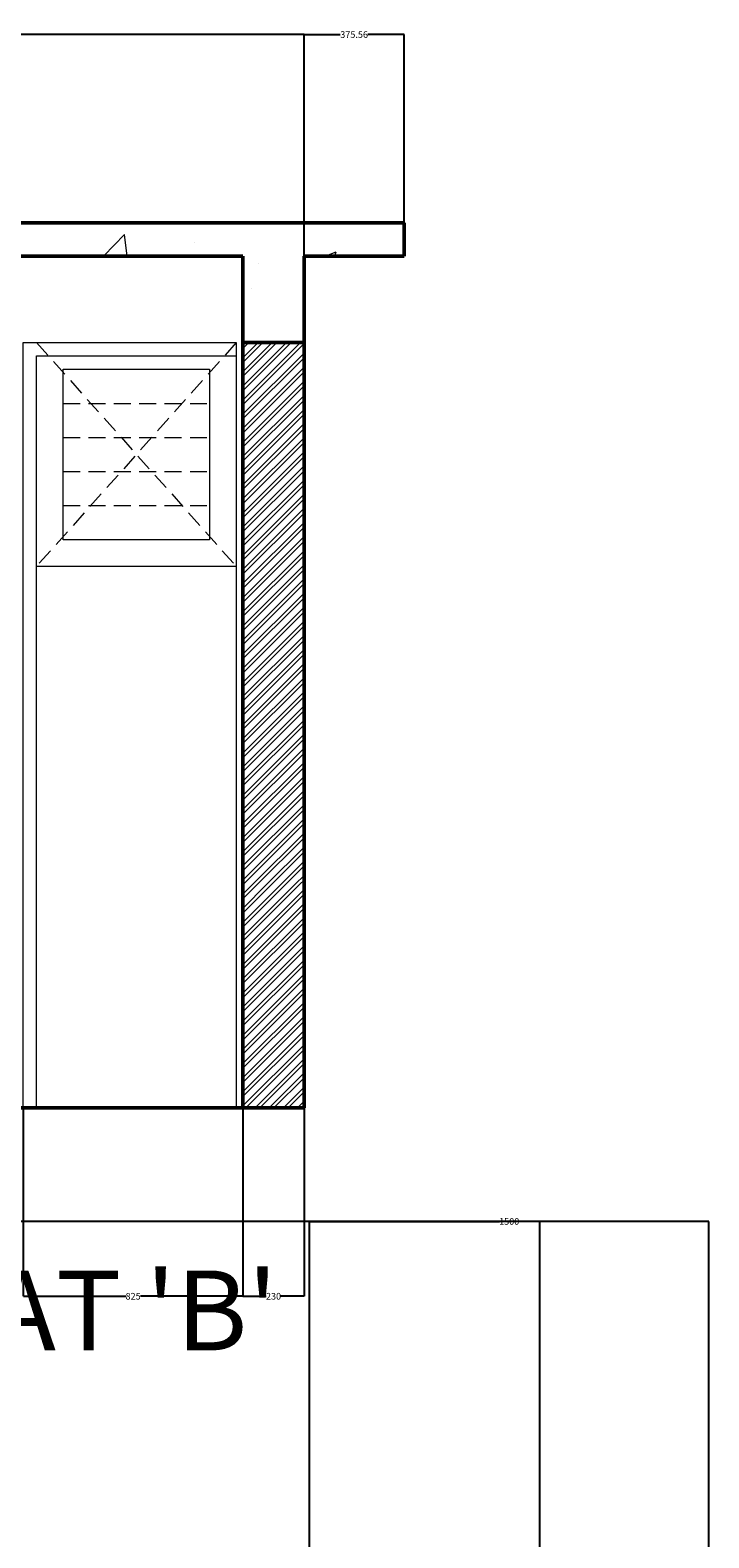
# Model space of a CAD drawing. Units: millimetres. Extents: x 1944 to 29915, y -10550 to 5909.
# Tile 24 of 24: x 23475 to 26024, y -1584 to 4080. Entities that reach past the tile are written whole.
import ezdxf

# ---------------------------------------------------------------- set-up
doc = ezdxf.new("R2010")
doc.units = ezdxf.units.MM
doc.header["$MEASUREMENT"] = 0
doc.linetypes.add('HIDDEN', pattern=[9.525, 6.35, -3.175])
for name, color, linetype, lineweight in [('A-ANNO-DIMS', 2, 'Continuous', 18), ('A-ANNO-TEXT', 7, 'Continuous', 25), ('A-ELEV', 3, 'Continuous', 18), ('A-ELEV-HIDN', 3, 'HIDDEN', 13), ('A-WALL', 7, 'Continuous', 50), ('A-WALL-PATT', 8, 'Continuous', 18)]:
    doc.layers.add(name, color=color, linetype=linetype, lineweight=lineweight)
doc.styles.get("Standard").update_dxf_attribs({"font": 'arial.ttf'})
doc.dimstyles.get("Standard").update_dxf_attribs({"dimtxt": 25, "dimasz": 0.18, "dimexe": 0.18, "dimexo": 0.0625, "dimgap": 0.09, "dimtad": 0, "dimtih": 1, "dimtoh": 1, "dimdec": 0, "dimzin": 0, "dimdsep": 46, "dimtxsty": 'Standard', "dimcen": 0.09, "dimadec": 0, "dimazin": 0, "dimtfac": 1, "dimtdec": 0, "dimtofl": 0, "dimtmove": 0, "dimatfit": 3, "dimfxl": 1, "dimtolj": 1, "dimtzin": 0, "dimarcsym": 0})

# ---------------------------------------------------------------- blocks, each defined once
blk = doc.blocks.new('*D73')
at = {"layer": 'A-ANNO-DIMS', "color": 0, "lineweight": -2, "transparency": 16777216}
for p, q in [((20250.9, 3230.9), (20250.9, 4063.5)), ((20251, 4063.3), (22339.6, 4063.3)), ((24504, 4063.3), (22415.4, 4063.3)), ((24504.1, 3230.9), (24504.1, 4063.5))]:
    blk.add_line(p, q, dxfattribs=at)
at = {"layer": 'A-ANNO-DIMS', "color": 0, "transparency": 16777216}
for points in [[(20251, 4063.4), (20251, 4063.3), (20250.9, 4063.3)], [(24504, 4063.4), (24504, 4063.3), (24504.1, 4063.3)]]:
    blk.add_solid(points, dxfattribs=at)
at = {"layer": 'Defpoints', "color": 0, "transparency": 16777216}
for p in [(24504.1, 4063.3), (20250.9, 3230.8), (24504.1, 3230.8)]:
    blk.add_point(p, dxfattribs=at)
at = {"layer": 'A-ANNO-DIMS', "color": 0, "transparency": 16777216, "insert": (22377.5, 4063.3), "char_height": 25, "attachment_point": 5}
blk.add_mtext('\\A1;4253', dxfattribs=at)
blk = doc.blocks.new('*D74')
at = {"layer": 'A-ANNO-DIMS', "color": 0, "lineweight": -2, "transparency": 16777216}
for p, q in [((24504.1, 3230.9), (24504.1, 4063.5)), ((24504.3, 4063.3), (24640, 4063.3)), ((24879.5, 4063.3), (24743.9, 4063.3)), ((24879.7, 3230.9), (24879.7, 4063.5))]:
    blk.add_line(p, q, dxfattribs=at)
at = {"layer": 'A-ANNO-DIMS', "color": 0, "transparency": 16777216}
for points in [[(24504.3, 4063.4), (24504.3, 4063.3), (24504.1, 4063.3)], [(24879.5, 4063.4), (24879.5, 4063.3), (24879.7, 4063.3)]]:
    blk.add_solid(points, dxfattribs=at)
at = {"layer": 'Defpoints', "color": 0, "transparency": 16777216}
for p in [(24879.7, 4063.3), (24504.1, 3230.8), (24879.7, 3230.8)]:
    blk.add_point(p, dxfattribs=at)
at = {"layer": 'A-ANNO-DIMS', "color": 0, "transparency": 16777216, "insert": (24691.9, 4063.3), "char_height": 25, "attachment_point": 5}
blk.add_mtext('\\A1;375.56', dxfattribs=at)
blk = doc.blocks.new('*D81')
at = {"layer": 'A-ANNO-DIMS', "color": 0, "lineweight": -2, "transparency": 16777216}
for p, q in [((23449.1, 30.8), (23449.1, -677)), ((24274.1, 30.8), (24274.1, -677)), ((23449.3, -676.8), (23833.8, -676.8)), ((24274, -676.8), (23889.5, -676.8))]:
    blk.add_line(p, q, dxfattribs=at)
at = {"layer": 'A-ANNO-DIMS', "color": 0, "transparency": 16777216}
for points in [[(23449.3, -676.8), (23449.3, -676.9), (23449.1, -676.8)], [(24274, -676.8), (24274, -676.9), (24274.1, -676.8)]]:
    blk.add_solid(points, dxfattribs=at)
at = {"layer": 'Defpoints', "color": 0, "transparency": 16777216}
for p in [(23449.1, 30.8), (24274.1, 30.8), (24274.1, -676.8)]:
    blk.add_point(p, dxfattribs=at)
at = {"layer": 'A-ANNO-DIMS', "color": 0, "transparency": 16777216, "insert": (23861.6, -676.8), "char_height": 25, "attachment_point": 5}
blk.add_mtext('\\A1;825', dxfattribs=at)
blk = doc.blocks.new('*D82')
at = {"layer": 'A-ANNO-DIMS', "color": 0, "lineweight": -2, "transparency": 16777216}
for p, q in [((24274.1, 30.8), (24274.1, -677)), ((24504.1, 30.8), (24504.1, -677)), ((24274.3, -676.8), (24361.3, -676.8)), ((24504, -676.8), (24417, -676.8))]:
    blk.add_line(p, q, dxfattribs=at)
at = {"layer": 'A-ANNO-DIMS', "color": 0, "transparency": 16777216}
for points in [[(24274.3, -676.8), (24274.3, -676.9), (24274.1, -676.8)], [(24504, -676.8), (24504, -676.9), (24504.1, -676.8)]]:
    blk.add_solid(points, dxfattribs=at)
at = {"layer": 'Defpoints', "color": 0, "transparency": 16777216}
for p in [(24274.1, 30.8), (24504.1, 30.8), (24504.1, -676.8)]:
    blk.add_point(p, dxfattribs=at)
at = {"layer": 'A-ANNO-DIMS', "color": 0, "transparency": 16777216, "insert": (24389.1, -676.8), "char_height": 25, "attachment_point": 5}
blk.add_mtext('\\A1;230', dxfattribs=at)
blk = doc.blocks.new('*D85')
at = {"layer": 'A-ANNO-DIMS', "color": 0, "lineweight": -2, "transparency": 16777216}
for p, q in [((6418.3, -1730.7), (6418.3, -395.6)), ((6418.5, -395.8), (15860.3, -395.8)), ((25389.1, -395.8), (15947.3, -395.8)), ((25389.3, -1846.5), (25389.3, -395.6))]:
    blk.add_line(p, q, dxfattribs=at)
at = {"layer": 'A-ANNO-DIMS', "color": 0, "transparency": 16777216}
for points in [[(6418.5, -395.7), (6418.5, -395.8), (6418.3, -395.8)], [(25389.1, -395.7), (25389.1, -395.8), (25389.3, -395.8)]]:
    blk.add_solid(points, dxfattribs=at)
at = {"layer": 'Defpoints', "color": 0, "transparency": 16777216}
for p in [(25389.3, -395.8), (6418.3, -1730.8), (25389.3, -1846.5)]:
    blk.add_point(p, dxfattribs=at)
at = {"layer": 'A-ANNO-DIMS', "color": 0, "transparency": 16777216, "insert": (15903.8, -395.8), "char_height": 25, "attachment_point": 5}
blk.add_mtext('\\A1;18971', dxfattribs=at)
blk = doc.blocks.new('*D91')
at = {"layer": 'A-ANNO-DIMS', "color": 0, "lineweight": -2, "transparency": 16777216}
for p, q in [((24524.3, -7516.2), (24524.3, -395.6)), ((24524.5, -395.8), (25238.1, -395.8)), ((26024.1, -395.8), (25310.5, -395.8)), ((26024.3, -7516.2), (26024.3, -395.6))]:
    blk.add_line(p, q, dxfattribs=at)
at = {"layer": 'A-ANNO-DIMS', "color": 0, "transparency": 16777216}
for points in [[(24524.5, -395.7), (24524.5, -395.8), (24524.3, -395.8)], [(26024.1, -395.7), (26024.1, -395.8), (26024.3, -395.8)]]:
    blk.add_solid(points, dxfattribs=at)
at = {"layer": 'Defpoints', "color": 0, "transparency": 16777216}
for p in [(26024.3, -395.8), (24524.3, -7516.2), (26024.3, -7516.2)]:
    blk.add_point(p, dxfattribs=at)
at = {"layer": 'A-ANNO-DIMS', "color": 0, "transparency": 16777216, "insert": (25274.3, -395.8), "char_height": 25, "attachment_point": 5}
blk.add_mtext('\\A1;1500', dxfattribs=at)

msp = doc.modelspace()

# ---------------------------------------------------------------- hatches: boundary and pattern name
at = {"layer": 'A-WALL-PATT'}
h = msp.add_hatch(dxfattribs=at)
h.set_pattern_fill('AR-CONC', color=256, scale=100)
h.paths.add_polyline_path([(24879.698, 3355.837), (20124.649, 3355.837), (20124.649, 3230.837), (20250.858, 3230.837), (20250.858, 2905.837), (20480.858, 2905.837), (20480.858, 3230.837), (24274.139, 3230.837), (24274.139, 2905.837), (24504.139, 2905.837), (24504.139, 3230.837), (24879.698, 3230.837)])
h = msp.add_hatch(dxfattribs=at)
h.set_pattern_fill('ANSI32', color=256, scale=100)
h.paths.add_polyline_path([(24504.139, 2905.837), (24274.139, 2905.837), (24274.139, 870.837), (24504.139, 870.837)])
h = msp.add_hatch(dxfattribs=at)
h.set_pattern_fill('ANSI32', color=256, scale=100)
h.paths.add_polyline_path([(24504.139, 870.837), (24274.139, 870.837), (24274.139, 30.837), (24504.139, 30.837)])

# ---------------------------------------------------------------- linework, layer by layer
at = {"layer": 'A-ELEV'}
for p, q in [((24249.139, 2905.837), (24249.139, 30.837)), ((24249.139, 2065.355), (23499.139, 2065.355))]:
    msp.add_line(p, q, dxfattribs=at)
for points in [[(23449.139, 30.837), (23449.139, 2905.837), (24249.139, 2905.837)], [(23499.139, 30.837), (23499.139, 2855.837), (24249.139, 2855.837)]]:
    msp.add_lwpolyline(points, dxfattribs=at)
msp.add_lwpolyline([(24149.139, 2805.837), (24149.139, 2165.355), (23599.139, 2165.355), (23599.139, 2805.837)], close=True, dxfattribs=at)
at = {"layer": 'A-ELEV-HIDN', "ltscale": 10}
for p, q in [((23499.139, 2905.837), (24249.139, 2065.355)), ((24249.139, 2905.837), (23499.139, 2065.355)), ((23599.139, 2677.741), (24149.139, 2677.741)), ((23599.139, 2549.644), (24149.139, 2549.644)), ((23599.139, 2421.548), (24149.139, 2421.548)), ((23599.139, 2293.451), (24149.139, 2293.451))]:
    msp.add_line(p, q, dxfattribs=at)
at = {"layer": 'A-WALL'}
for p, q in [((20124.649, 3355.837), (24879.698, 3355.837)), ((24879.698, 3355.837), (24879.698, 3230.837)), ((20480.858, 3230.837), (24274.139, 3230.837)), ((24274.139, 3230.837), (24274.139, 30.837)), ((24504.139, 3230.837), (24504.139, 30.837)), ((24504.139, 3230.837), (24879.698, 3230.837)), ((24274.139, 2905.837), (24504.139, 2905.837)), ((24504.139, 30.837), (12776.548, 30.837))]:
    msp.add_line(p, q, dxfattribs=at)

# ---------------------------------------------------------------- texts
at = {"layer": 'A-ANNO-TEXT'}
msp.add_text("SECTION AT 'B'", height=300, dxfattribs=at).set_placement((21520.494, -880.236))

# ---------------------------------------------------------------- dimensions: what is measured, and where the dimension line sits
at = {"layer": 'A-ANNO-DIMS'}
for base, p1, p2, override, picture, middle in [((24504.139, 4063.337), (20250.858, 3230.837), (24504.139, 3230.837), {"dimdec": 0, "dimlfac": 1, "dimrnd": 0, "dimzin": 0, "dimdsep": 46, "dimlunit": 2}, '*D73', (22377.499, 4063.337)), ((24879.698, 4063.337), (24504.139, 3230.837), (24879.698, 3230.837), {"dimdec": 2, "dimlfac": 1, "dimrnd": 0, "dimzin": 0, "dimdsep": 46, "dimlunit": 2}, '*D74', (24691.919, 4063.337)), ((24274.139, -676.843), (23449.139, 30.837), (24274.139, 30.837), {"dimdec": 0, "dimlfac": 1, "dimrnd": 0, "dimzin": 0, "dimdsep": 46, "dimlunit": 2}, '*D81', (23861.639, -676.843)), ((24504.139, -676.843), (24274.139, 30.837), (24504.139, 30.837), {"dimdec": 0, "dimlfac": 1, "dimrnd": 0, "dimzin": 0, "dimdsep": 46, "dimlunit": 2}, '*D82', (24389.139, -676.843)), ((25389.297, -395.752), (6418.315, -1730.752), (25389.297, -1846.542), {"dimdec": 0, "dimlfac": 1, "dimrnd": 0, "dimzin": 0, "dimdsep": 46, "dimlunit": 2}, '*D85', (15903.806, -395.752)), ((26024.297, -395.752), (24524.297, -7516.218), (26024.297, -7516.218), {"dimdec": 0, "dimlfac": 1, "dimrnd": 0, "dimzin": 0, "dimdsep": 46, "dimlunit": 2}, '*D91', (25274.297, -395.752))]:
    dim = msp.add_linear_dim(base=base, p1=p1, p2=p2, dimstyle='Standard', override=override, dxfattribs=at)
    dim.commit()
    dim.dimension.update_dxf_attribs({"geometry": picture, "text_midpoint": middle})

doc.saveas('drawing.dxf')
